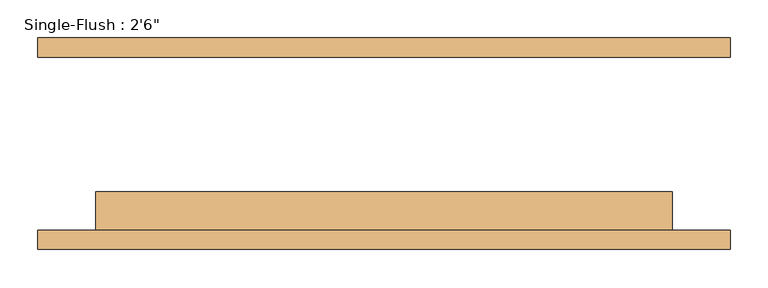
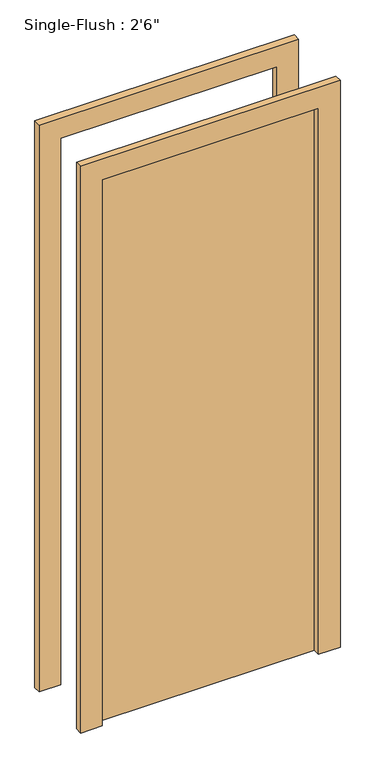
"""IFC4 building model written with IfcOpenShell, lengths in millimetres: door geometry."""

from ifc_helpers import new_model, si_unit, frame, origin, origin_with_axes, place, context, project, spatial, polyline, outline, extrude, source, transform, mapped, element, save


def door_85036156(model_context):
    return source(origin(), model_context, "Body", "SweptSolid", [
        extrude(outline(polyline([(2108.2, -457.2), (0.0, -457.2), (0.0, -381.0), (2032.0, -381.0), (2032.0, 381.0), (0.0, 381.0), (0.0, 457.2), (2108.2, 457.2), (2108.2, -457.2)])), frame((0.0, -139.7, 0.0), z_axis=(0.0, 1.0, 0.0), x_axis=(0.0, 0.0, 1.0)), (0.0, 0.0, 1.0), 25.4),
        extrude(outline(polyline([(2108.2, 457.2), (2108.2, -457.2), (0.0, -457.2), (0.0, -381.0), (2032.0, -381.0), (2032.0, 381.0), (0.0, 381.0), (0.0, 457.2), (2108.2, 457.2)])), frame((0.0, 114.3, 0.0), z_axis=(0.0, 1.0, 0.0), x_axis=(0.0, 0.0, 1.0)), (0.0, 0.0, 1.0), 25.4),
        extrude(outline(polyline([(381.0, -63.5), (381.0, -114.3), (-381.0, -114.3), (-381.0, -63.5), (381.0, -63.5)])), origin_with_axes(), (0.0, 0.0, 1.0), 2032.0),
    ])


if __name__ == "__main__":
    model = new_model("IFC4")
    model_context = context("Model", 3, world=origin())
    ifc_project = project(units=[si_unit("LENGTHUNIT", "METRE", prefix="MILLI")], contexts=[model_context])
    site = spatial("IfcSite", under=ifc_project)
    building = spatial("IfcBuilding", under=site)
    placement = place(None, origin())
    door_shape = door_85036156(model_context)
    element("IfcDoor", 1, ObjectType="Single-Flush : 2'6\"", at=placement, inside=building, context=model_context, shape_type="MappedRepresentation", body=[
        mapped(door_shape, transform((0.0, 0.0, 0.0), x_axis=(1.0, 0.0, 0.0), y_axis=(0.0, 1.0, 0.0), z_axis=(0.0, 0.0, 1.0))),
    ])
    save(model, "model.ifc")

# Revit data of these elements
# Type "Single-Flush : 2'6\""
#   Type Mark = "14"
#   Construction Type Id = "MDOOR"
#   Assembly Code = "C1020"
#   Analytic Construction = "Metal"
#   Rough Width = 2' - 6"
#   Rough Height = 7' - 0"
#   Thickness = 0' - 2"
#   Heat Transfer Coefficient (U) = 0.651978 BTU/(h·ft²·°F)
#   Height = 6' - 8"
#   Trim Projection Ext = 0' - 1"
#   Trim Projection Int = 0' - 1"
#   Trim Width = 0' - 3"
#   Width = 2' - 6"
#   Define Thermal Properties by = 1
#   Door Material = Door - Panel
#   Frame Material = Door - Frame
#   Visual Light Transmittance = 0
#   Solar Heat Gain Coefficient = 0
#   Function = (empty or 0)
#   Wall Closure = (empty or 0)
# Element 1 (IfcDoor, "Single-Flush : 2'6\"")
#   Materials on its faces: "Door - Frame", "Door - Panel"
# Materials
#   "Door - Panel": class "Wood", colour RGB 210 159 95, transparency 0, Cost = 0
#   "Door - Frame": colour RGB 118 70 51, transparency 0, Cost = 0
